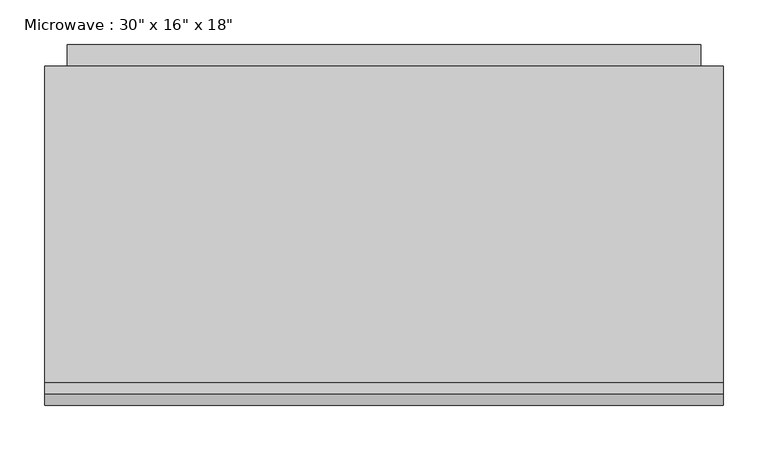
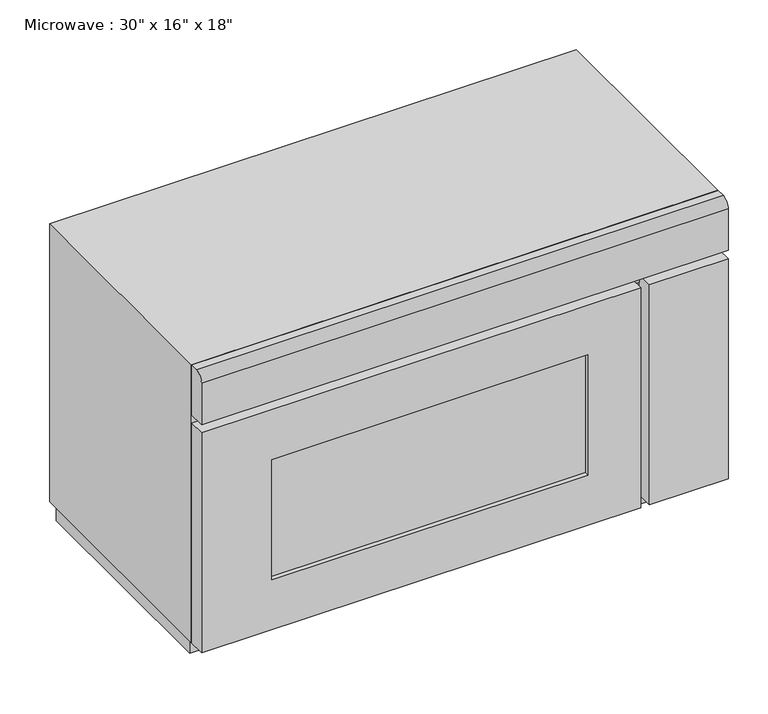
"""IFC4 building model written with IfcOpenShell, lengths in millimetres: proxy geometry."""

from ifc_helpers import new_model, si_unit, point, frame, frame_2d, origin, place, context, project, spatial, polyline, circle_curve, trimmed, segment, composite_curve, outline, extrude, faceted_brep, source, transform, mapped, element, save


def proxy_e661f726(model_context):
    return source(origin(), model_context, "Body", "SolidModel", [
        extrude(outline(polyline([(871.7678773, -175.2805058), (871.7678773, -510.2430058), (128.8178773, -510.2430058), (128.8178773, -175.2805058), (871.7678773, -175.2805058)])), frame((0.0, 0.0, 914.4), z_axis=(0.0, 0.0, 1.0), x_axis=(1.0, 0.0, 0.0)), (0.0, 0.0, 1.0), 31.75),
        faceted_brep([(881.2928773, -175.2805058, 1371.6), (119.2928773, -175.2805058, 1371.6), (119.2928773, -530.8805058, 1371.6), (881.2928773, -530.8805058, 1371.6), (881.2928773, -175.2805058, 946.15), (881.2928773, -530.8805058, 946.15), (119.2928773, -530.8805058, 946.15), (119.2928773, -175.2805058, 946.15), (824.5397523, -530.8805058, 1271.0014904), (824.5397523, -530.8805058, 1020.1764904), (176.0460023, -530.8805058, 1020.1764904), (176.0460023, -530.8805058, 1271.0014904), (824.5397523, -200.6805058, 1271.0014904), (176.0460023, -200.6805058, 1271.0014904), (176.0460023, -200.6805058, 1020.1764904), (824.5397523, -200.6805058, 1020.1764904)], [[[0, 1, 2, 3]], [[4, 5, 6, 7]], [[1, 0, 4, 7]], [[2, 1, 7, 6]], [[3, 2, 6, 5], [8, 9, 10, 11]], [[0, 3, 5, 4]], [[12, 13, 14, 15]], [[12, 15, 9, 8]], [[15, 14, 10, 9]], [[14, 13, 11, 10]], [[13, 12, 8, 11]]]),
        extrude(outline(polyline([(-151.0441495, 1346.2), (-151.0441495, 961.946551), (-176.4441495, 936.546551), (-176.4441495, 1346.2), (-151.0441495, 1346.2)])), frame((144.6928773, 0.0, 0.0), z_axis=(1.0, 0.0, 0.0), x_axis=(0.0, 1.0, 0.0)), (0.0, 0.0, 1.0), 711.2),
        extrude(outline(composite_curve([segment(polyline([(-543.5805058, 1371.6), (-530.8805058, 1371.6), (-530.8805058, 1295.4), (-556.2805058, 1295.4), (-556.2805058, 1358.9)]), True, "CONTINUOUS"), segment(trimmed(circle_curve(frame_2d((-543.5805058, 1358.9)), 12.7), [point((-556.2805058, 1358.9))], [point((-543.5805058, 1371.6))], False, "CARTESIAN"), True, "CONTINUOUS")], self_intersect=False)), frame((119.2928773, 0.0, 0.0), z_axis=(1.0, 0.0, 0.0), x_axis=(0.0, 1.0, 0.0)), (0.0, 0.0, 1.0), 762.0),
        extrude(outline(polyline([(1282.7, 754.6897523), (1282.7, 119.2928773), (946.15, 119.2928773), (946.15, 754.6897523), (1282.7, 754.6897523)]), holes=[polyline([(1206.5, 678.4897523), (1022.35, 678.4897523), (1022.35, 220.8928773), (1206.5, 220.8928773), (1206.5, 678.4897523)])]), frame((0.0, -556.2805058, 0.0), z_axis=(0.0, 1.0, 0.0), x_axis=(0.0, 0.0, 1.0)), (0.0, 0.0, 1.0), 25.4),
        extrude(outline(polyline([(881.2928773, -556.2805058), (767.3897523, -556.2805058), (767.3897523, -530.8805058), (881.2928773, -530.8805058), (881.2928773, -556.2805058)])), frame((0.0, 0.0, 946.15), z_axis=(0.0, 0.0, 1.0), x_axis=(1.0, 0.0, 0.0)), (0.0, 0.0, 1.0), 336.55),
        extrude(outline(polyline([(678.4897523, -549.9305058), (220.8928773, -549.9305058), (220.8928773, -543.5805058), (678.4897523, -543.5805058), (678.4897523, -549.9305058)])), frame((0.0, 0.0, 1022.35), z_axis=(0.0, 0.0, 1.0), x_axis=(1.0, 0.0, 0.0)), (0.0, 0.0, 1.0), 184.15),
    ])


if __name__ == "__main__":
    model = new_model("IFC4")
    model_context = context("Model", 3, world=origin())
    ifc_project = project(units=[si_unit("LENGTHUNIT", "METRE", prefix="MILLI")], contexts=[model_context])
    site = spatial("IfcSite", under=ifc_project)
    building = spatial("IfcBuilding", under=site)
    placement = place(None, origin())
    proxy_shape = proxy_e661f726(model_context)
    element("IfcBuildingElementProxy", 1, Name="Microwave : 30\" x 16\" x 18\"", ObjectType="Microwave : 30\" x 16\" x 18\"", at=placement, inside=building, context=model_context, shape_type="MappedRepresentation", body=[
        mapped(proxy_shape, transform((0.0, 0.0, 0.0), x_axis=(1.0, 0.0, 0.0), y_axis=(0.0, 1.0, 0.0), z_axis=(0.0, 0.0, 1.0))),
    ])
    save(model, "model.ifc")

# Revit data of these elements
# Type "Microwave : 30\" x 16\" x 18\""
#   Assembly Code = "E1090400"
#   Depth = 1' - 4"
#   Height = 1' - 6"
#   Width = 2' - 6"
#   Microwave Material = Laminate - Ivory,Matte
#   Default Elevation = 0
# Element 1 (IfcBuildingElementProxy, "Microwave : 30\" x 16\" x 18\"")
#   Materials on its faces: "Laminate - Ivory,Matte", "Glass"
# Materials
#   "Laminate - Ivory,Matte": colour RGB 247 247 239, transparency 0
#   "Glass": class "Glass", colour RGB 0 128 192, transparency 0.75, Description = "Soda Lime Glass", Cost = 0
